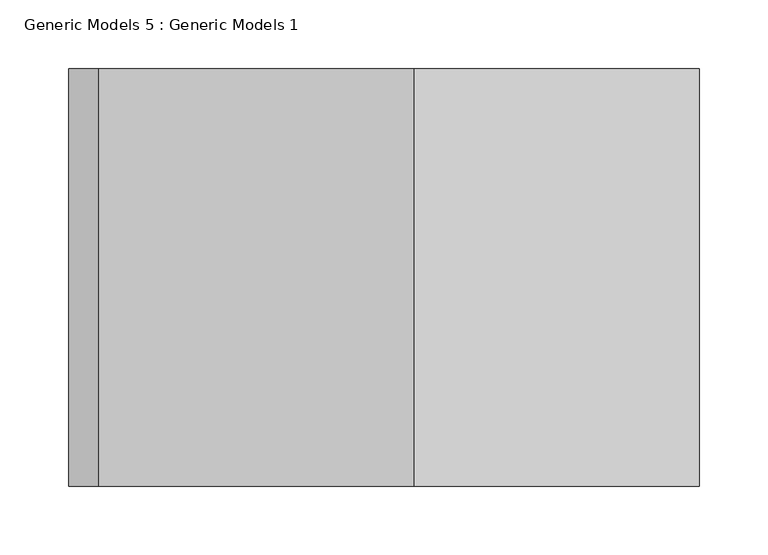
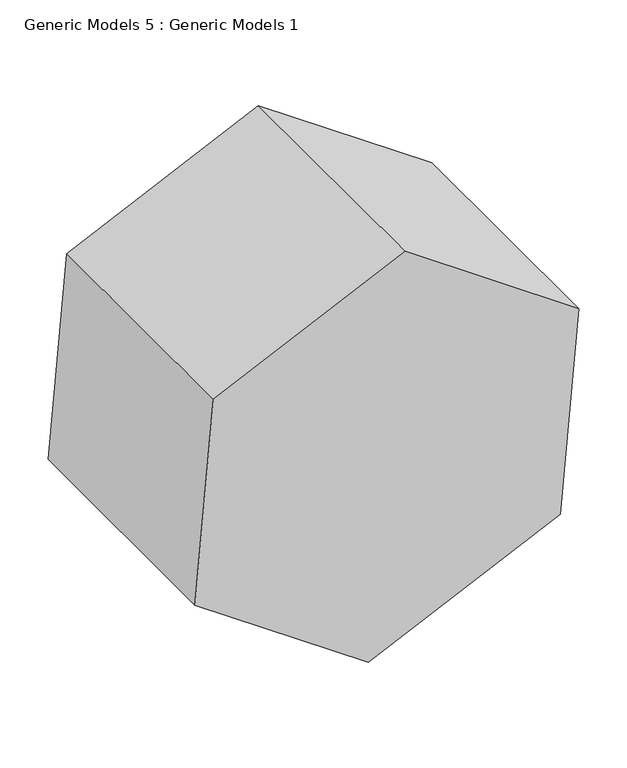
"""IFC4 building model written with IfcOpenShell, lengths in millimetres: proxy geometry, Generic Models 5 : Generic Models 1."""

from ifc_helpers import new_model, si_unit, frame, origin, place, context, project, spatial, polyline, outline, extrude, source, transform, mapped, element, save


def generic_models_5_generic_models_1_6c1de215(model_context):
    return source(origin(), model_context, "Body", "SweptSolid", [
        extrude(outline(polyline([(833.1013393, -4219.9079055), (978.7897542, -4427.9725247), (871.4447157, -4658.1747026), (618.4112624, -4680.3122613), (472.7228475, -4472.247642), (580.067886, -4242.0454641), (833.1013393, -4219.9079055)])), frame((0.0, -10720.3372434, 0.0), z_axis=(0.0, 1.0, 0.0), x_axis=(0.0, 0.0, 1.0)), (0.0, 0.0, 1.0), 304.8),
    ])


if __name__ == "__main__":
    model = new_model("IFC4")
    model_context = context("Model", 3, world=origin())
    ifc_project = project(units=[si_unit("LENGTHUNIT", "METRE", prefix="MILLI")], contexts=[model_context])
    site = spatial("IfcSite", under=ifc_project)
    building = spatial("IfcBuilding", under=site)
    placement = place(None, origin())
    generic_models_5_generic_models_1_shape = generic_models_5_generic_models_1_6c1de215(model_context)
    element("IfcBuildingElementProxy", 1, Name="Generic Models 5 : Generic Models 1", ObjectType="Generic Models 5 : Generic Models 1", at=placement, inside=building, context=model_context, shape_type="MappedRepresentation", body=[
        mapped(generic_models_5_generic_models_1_shape, transform((0.0, 0.0, 0.0), x_axis=(1.0, 0.0, 0.0), y_axis=(0.0, 1.0, 0.0), z_axis=(0.0, 0.0, 1.0))),
    ])
    save(model, "model.ifc")

# Revit data of these elements
# Element 1 (IfcBuildingElementProxy, "Generic Models 5 : Generic Models 1")
#   Materials on its faces: "Render Material 41-165-0"
# Materials
#   "Render Material 41-165-0": colour RGB 41 165 0, transparency 0
